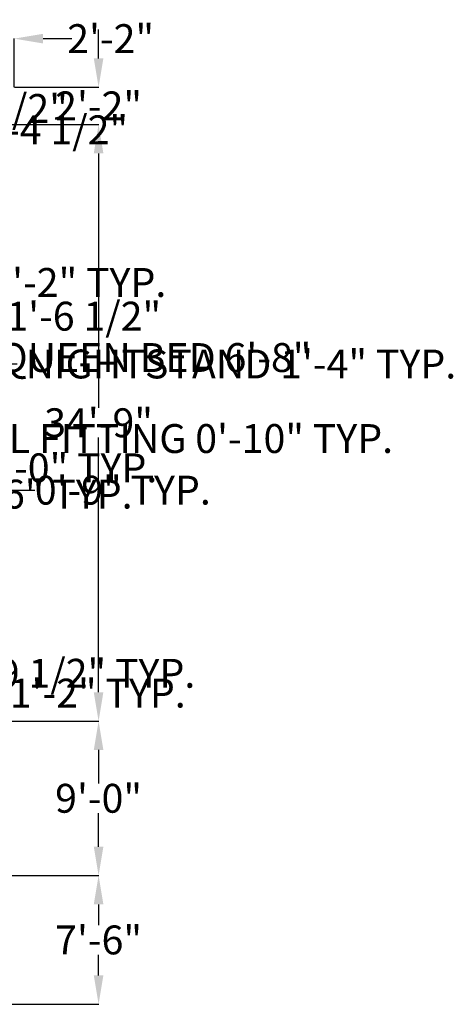
# Model space of a CAD drawing. Units: inches. Extents: x 1202 to 2101, y 998 to 1743.
# Tile 4 of 4: x 1798 to 2101, y 1054 to 1743. Entities that reach past the tile are written whole.
import ezdxf

# ---------------------------------------------------------------- set-up
doc = ezdxf.new("R2010")
doc.units = ezdxf.units.IN
doc.header["$MEASUREMENT"] = 0
doc.layers.add('A-ANNO-DIMS', color=2, linetype='Continuous', lineweight=18)
doc.styles.get("Standard").update_dxf_attribs({"font": 'arial.ttf'})
doc.dimstyles.get("Standard").update_dxf_attribs({"dimtxt": 20.18, "dimasz": 20.18, "dimexe": 0.18, "dimexo": 0.0625, "dimgap": 0.09, "dimtad": 0, "dimtih": 1, "dimtoh": 1, "dimdec": 0, "dimzin": 0, "dimdsep": 46, "dimlunit": 3, "dimtxsty": 'Standard', "dimcen": 0.09, "dimadec": 0, "dimazin": 0, "dimtfac": 1, "dimtdec": 0, "dimtofl": 0, "dimtmove": 0, "dimatfit": 3, "dimfxl": 1, "dimtolj": 1, "dimtzin": 0, "dimarcsym": 0})

# ---------------------------------------------------------------- blocks, each defined once
blk = doc.blocks.new('*D21')
at = {"layer": 'A-ANNO-DIMS', "color": 0, "lineweight": -2, "transparency": 16777216}
for p, q in [((1771.58, 1461.65), (1771.58, 1481.83)), ((1768.04, 1441.47), (1771.76, 1441.47)), ((1768.04, 1417.47), (1771.76, 1417.47)), ((1771.58, 1397.29), (1771.58, 1377.11))]:
    blk.add_line(p, q, dxfattribs=at)
at = {"layer": 'A-ANNO-DIMS', "color": 0, "transparency": 16777216}
for points in [[(1768.21, 1461.65), (1774.94, 1461.65), (1771.58, 1441.47)], [(1768.21, 1397.29), (1774.94, 1397.29), (1771.58, 1417.47)]]:
    blk.add_solid(points, dxfattribs=at)
at = {"layer": 'Defpoints', "color": 0, "transparency": 16777216}
for p in [(1767.98, 1441.47), (1771.58, 1441.47), (1767.98, 1417.47)]:
    blk.add_point(p, dxfattribs=at)
at = {"layer": 'A-ANNO-DIMS', "color": 0, "transparency": 16777216, "insert": (1771.58, 1429.47), "char_height": 20.18, "attachment_point": 5}
blk.add_mtext('\\A1;WINDOW 2\'-0" TYP.', dxfattribs=at)
blk = doc.blocks.new('*D22')
at = {"layer": 'A-ANNO-DIMS', "color": 0, "lineweight": -2, "transparency": 16777216}
for p, q in [((1738.8, 1413.87), (1718.62, 1413.87)), ((1758.98, 1417.4), (1758.98, 1413.69)), ((1767.98, 1417.4), (1767.98, 1413.69)), ((1788.16, 1413.87), (1808.34, 1413.87))]:
    blk.add_line(p, q, dxfattribs=at)
at = {"layer": 'A-ANNO-DIMS', "color": 0, "transparency": 16777216}
for points in [[(1738.8, 1417.23), (1738.8, 1410.5), (1758.98, 1413.87)], [(1788.16, 1417.23), (1788.16, 1410.5), (1767.98, 1413.87)]]:
    blk.add_solid(points, dxfattribs=at)
at = {"layer": 'Defpoints', "color": 0, "transparency": 16777216}
for p in [(1758.98, 1417.47), (1767.98, 1417.47), (1767.98, 1413.87)]:
    blk.add_point(p, dxfattribs=at)
at = {"layer": 'A-ANNO-DIMS', "color": 0, "transparency": 16777216, "insert": (1869.93, 1413.87), "char_height": 20.18, "attachment_point": 5}
blk.add_mtext('\\A1;0\'-9" TYP.', dxfattribs=at)
blk = doc.blocks.new('*D23')
at = {"layer": 'A-ANNO-DIMS', "color": 0, "lineweight": -2, "transparency": 16777216}
for p, q in [((1705.63, 1429.75), (1705.63, 1449.93)), ((1705.63, 1449.93), (1725.81, 1449.93)), ((1707.09, 1409.57), (1705.45, 1409.57)), ((1707.09, 1399.47), (1705.45, 1399.47)), ((1705.63, 1379.29), (1705.63, 1359.11))]:
    blk.add_line(p, q, dxfattribs=at)
at = {"layer": 'A-ANNO-DIMS', "color": 0, "transparency": 16777216}
for points in [[(1702.27, 1429.75), (1709, 1429.75), (1705.63, 1409.57)], [(1702.27, 1379.29), (1709, 1379.29), (1705.63, 1399.47)]]:
    blk.add_solid(points, dxfattribs=at)
at = {"layer": 'Defpoints', "color": 0, "transparency": 16777216}
for p in [(1705.63, 1409.57), (1707.15, 1409.57), (1707.15, 1399.47)]:
    blk.add_point(p, dxfattribs=at)
at = {"layer": 'A-ANNO-DIMS', "color": 0, "transparency": 16777216, "insert": (1896.68, 1449.93), "char_height": 20.18, "attachment_point": 5}
blk.add_mtext('\\A1;WALL FITTING 0\'-10" TYP.', dxfattribs=at)
blk = doc.blocks.new('*D24')
at = {"layer": 'A-ANNO-DIMS', "color": 0, "lineweight": -2, "transparency": 16777216}
for p, q in [((1686.97, 1411.09), (1666.79, 1411.09)), ((1707.15, 1409.64), (1707.15, 1411.27)), ((1713.22, 1409.64), (1713.22, 1411.27)), ((1733.4, 1411.09), (1753.58, 1411.09))]:
    blk.add_line(p, q, dxfattribs=at)
at = {"layer": 'A-ANNO-DIMS', "color": 0, "transparency": 16777216}
for points in [[(1686.97, 1414.45), (1686.97, 1407.73), (1707.15, 1411.09)], [(1733.4, 1414.45), (1733.4, 1407.73), (1713.22, 1411.09)]]:
    blk.add_solid(points, dxfattribs=at)
at = {"layer": 'Defpoints', "color": 0, "transparency": 16777216}
for p in [(1713.22, 1411.09), (1707.15, 1409.57), (1713.22, 1409.57)]:
    blk.add_point(p, dxfattribs=at)
at = {"layer": 'A-ANNO-DIMS', "color": 0, "transparency": 16777216, "insert": (1815.17, 1411.09), "char_height": 20.18, "attachment_point": 5}
blk.add_mtext('\\A1;0\'-6" TYP.', dxfattribs=at)
blk = doc.blocks.new('*D25')
at = {"layer": 'A-ANNO-DIMS', "color": 0, "lineweight": -2, "transparency": 16777216}
for p, q in [((1754.58, 1316.69), (1754.58, 1336.87)), ((1751.44, 1296.51), (1754.76, 1296.51)), ((1751.44, 1275.18), (1754.76, 1275.18)), ((1754.58, 1255), (1754.58, 1234.82))]:
    blk.add_line(p, q, dxfattribs=at)
at = {"layer": 'A-ANNO-DIMS', "color": 0, "transparency": 16777216}
for points in [[(1751.22, 1316.69), (1757.94, 1316.69), (1754.58, 1296.51)], [(1751.22, 1255), (1757.94, 1255), (1754.58, 1275.18)]]:
    blk.add_solid(points, dxfattribs=at)
at = {"layer": 'Defpoints', "color": 0, "transparency": 16777216}
for p in [(1751.38, 1296.51), (1754.58, 1296.51), (1751.38, 1275.18)]:
    blk.add_point(p, dxfattribs=at)
at = {"layer": 'A-ANNO-DIMS', "color": 0, "transparency": 16777216, "insert": (1754.58, 1285.85), "char_height": 20.18, "attachment_point": 5}
blk.add_mtext('\\A1;PILLOW SET 1\'-9 1/2" TYP.', dxfattribs=at)
blk = doc.blocks.new('*D26')
at = {"layer": 'A-ANNO-DIMS', "color": 0, "lineweight": -2, "transparency": 16777216}
for p, q in [((1737.22, 1275.12), (1737.22, 1271.8)), ((1751.38, 1275.12), (1751.38, 1271.8)), ((1717.04, 1271.98), (1696.86, 1271.98)), ((1771.56, 1271.98), (1791.74, 1271.98))]:
    blk.add_line(p, q, dxfattribs=at)
at = {"layer": 'A-ANNO-DIMS', "color": 0, "transparency": 16777216}
for points in [[(1717.04, 1275.35), (1717.04, 1268.62), (1737.22, 1271.98)], [(1771.56, 1275.35), (1771.56, 1268.62), (1751.38, 1271.98)]]:
    blk.add_solid(points, dxfattribs=at)
at = {"layer": 'Defpoints', "color": 0, "transparency": 16777216}
for p in [(1737.22, 1275.18), (1751.38, 1275.18), (1751.38, 1271.98)]:
    blk.add_point(p, dxfattribs=at)
at = {"layer": 'A-ANNO-DIMS', "color": 0, "transparency": 16777216, "insert": (1852.38, 1271.98), "char_height": 20.18, "attachment_point": 5}
blk.add_mtext('\\A1;1\'-2" TYP.', dxfattribs=at)
blk = doc.blocks.new('*D27')
at = {"layer": 'A-ANNO-DIMS', "color": 0, "lineweight": -2, "transparency": 16777216}
for p, q in [((1719.4, 1502.04), (1699.22, 1502.04)), ((1739.58, 1504.38), (1739.58, 1501.86)), ((1755.58, 1504.38), (1755.58, 1501.86)), ((1775.76, 1502.04), (1795.94, 1502.04))]:
    blk.add_line(p, q, dxfattribs=at)
at = {"layer": 'A-ANNO-DIMS', "color": 0, "transparency": 16777216}
for points in [[(1719.4, 1505.41), (1719.4, 1498.68), (1739.58, 1502.04)], [(1775.76, 1505.41), (1775.76, 1498.68), (1755.58, 1502.04)]]:
    blk.add_solid(points, dxfattribs=at)
at = {"layer": 'Defpoints', "color": 0, "transparency": 16777216}
for p in [(1739.58, 1504.44), (1755.58, 1504.44), (1755.58, 1502.04)]:
    blk.add_point(p, dxfattribs=at)
at = {"layer": 'A-ANNO-DIMS', "color": 0, "transparency": 16777216, "insert": (1952.58, 1502.04), "char_height": 20.18, "attachment_point": 5}
blk.add_mtext('\\A1;NIGHTSTAND 1\'-4" TYP.', dxfattribs=at)
blk = doc.blocks.new('*D28')
at = {"layer": 'A-ANNO-DIMS', "color": 0, "lineweight": -2, "transparency": 16777216}
for p, q in [((1757.98, 1538.86), (1757.98, 1559.04)), ((1757.98, 1559.04), (1778.16, 1559.04)), ((1755.64, 1518.68), (1758.16, 1518.68)), ((1755.64, 1504.44), (1758.16, 1504.44)), ((1757.98, 1484.26), (1757.98, 1464.08))]:
    blk.add_line(p, q, dxfattribs=at)
at = {"layer": 'A-ANNO-DIMS', "color": 0, "transparency": 16777216}
for points in [[(1754.62, 1538.86), (1761.34, 1538.86), (1757.98, 1518.68)], [(1754.62, 1484.26), (1761.34, 1484.26), (1757.98, 1504.44)]]:
    blk.add_solid(points, dxfattribs=at)
at = {"layer": 'Defpoints', "color": 0, "transparency": 16777216}
for p in [(1755.58, 1518.68), (1757.98, 1518.68), (1755.58, 1504.44)]:
    blk.add_point(p, dxfattribs=at)
at = {"layer": 'A-ANNO-DIMS', "color": 0, "transparency": 16777216, "insert": (1838.8, 1559.04), "char_height": 20.18, "attachment_point": 5}
blk.add_mtext('\\A1;1\'-2" TYP.', dxfattribs=at)
blk = doc.blocks.new('*D29')
at = {"layer": 'A-ANNO-DIMS', "color": 0, "lineweight": -2, "transparency": 16777216}
for p, q in [((1678.41, 1518.49), (1678.41, 1506.37)), ((1758.41, 1518.49), (1758.41, 1506.37)), ((1698.59, 1506.55), (1738.23, 1506.55)), ((1758.41, 1506.55), (1778.59, 1506.55))]:
    blk.add_line(p, q, dxfattribs=at)
at = {"layer": 'A-ANNO-DIMS', "color": 0, "transparency": 16777216}
for points in [[(1698.59, 1509.91), (1698.59, 1503.18), (1678.41, 1506.55)], [(1738.23, 1509.91), (1738.23, 1503.18), (1758.41, 1506.55)]]:
    blk.add_solid(points, dxfattribs=at)
at = {"layer": 'Defpoints', "color": 0, "transparency": 16777216}
for p in [(1678.41, 1518.55), (1758.41, 1518.55), (1758.41, 1506.55)]:
    blk.add_point(p, dxfattribs=at)
at = {"layer": 'A-ANNO-DIMS', "color": 0, "transparency": 16777216, "insert": (1892.42, 1506.55), "char_height": 20.18, "attachment_point": 5}
blk.add_mtext('\\A1;QUEEN BED 6\'-8"', dxfattribs=at)
blk = doc.blocks.new('*D37')
at = {"layer": 'A-ANNO-DIMS', "color": 0, "lineweight": -2, "transparency": 16777216}
for p, q in [((1628.63, 1659.71), (1628.63, 1665.93)), ((1648.81, 1665.75), (1649.15, 1665.75)), ((1669.33, 1659.71), (1669.33, 1665.93)), ((1669.33, 1665.75), (1689.51, 1665.75))]:
    blk.add_line(p, q, dxfattribs=at)
at = {"layer": 'A-ANNO-DIMS', "color": 0, "transparency": 16777216}
for points in [[(1648.81, 1669.11), (1648.81, 1662.39), (1628.63, 1665.75)], [(1649.15, 1669.11), (1649.15, 1662.39), (1669.33, 1665.75)]]:
    blk.add_solid(points, dxfattribs=at)
at = {"layer": 'Defpoints', "color": 0, "transparency": 16777216}
for p in [(1669.33, 1665.75), (1628.63, 1659.65), (1669.33, 1659.65)]:
    blk.add_point(p, dxfattribs=at)
at = {"layer": 'A-ANNO-DIMS', "color": 0, "transparency": 16777216, "insert": (1781.74, 1665.75), "char_height": 20.18, "attachment_point": 5}
blk.add_mtext('\\A1;DESK 3\'-4 1/2"', dxfattribs=at)
blk = doc.blocks.new('*D41')
at = {"layer": 'A-ANNO-DIMS', "color": 0, "lineweight": -2, "transparency": 16777216}
for p, q in [((1618.04, 1252.47), (1853.16, 1252.47)), ((1852.98, 1232.29), (1852.98, 1208.86)), ((1852.98, 1164.65), (1852.98, 1188.07)), ((1759.04, 1144.47), (1853.16, 1144.47))]:
    blk.add_line(p, q, dxfattribs=at)
at = {"layer": 'A-ANNO-DIMS', "color": 0, "transparency": 16777216}
for points in [[(1849.61, 1232.29), (1856.34, 1232.29), (1852.98, 1252.47)], [(1849.61, 1164.65), (1856.34, 1164.65), (1852.98, 1144.47)]]:
    blk.add_solid(points, dxfattribs=at)
at = {"layer": 'Defpoints', "color": 0, "transparency": 16777216}
for p in [(1617.98, 1252.47), (1852.98, 1252.47), (1758.98, 1144.47)]:
    blk.add_point(p, dxfattribs=at)
at = {"layer": 'A-ANNO-DIMS', "color": 0, "transparency": 16777216, "insert": (1852.98, 1198.47), "char_height": 20.18, "attachment_point": 5}
blk.add_mtext('\\A1;9\'-0"', dxfattribs=at)
blk = doc.blocks.new('*D42')
at = {"layer": 'A-ANNO-DIMS', "color": 0, "lineweight": -2, "transparency": 16777216}
for p, q in [((1768.04, 1669.47), (1853.16, 1669.47)), ((1852.98, 1649.29), (1852.98, 1471.37)), ((1852.98, 1272.65), (1852.98, 1450.57)), ((1618.04, 1252.47), (1853.16, 1252.47))]:
    blk.add_line(p, q, dxfattribs=at)
at = {"layer": 'A-ANNO-DIMS', "color": 0, "transparency": 16777216}
for points in [[(1849.61, 1649.29), (1856.34, 1649.29), (1852.98, 1669.47)], [(1849.61, 1272.65), (1856.34, 1272.65), (1852.98, 1252.47)]]:
    blk.add_solid(points, dxfattribs=at)
at = {"layer": 'Defpoints', "color": 0, "transparency": 16777216}
for p in [(1767.98, 1669.47), (1852.98, 1669.47), (1617.98, 1252.47)]:
    blk.add_point(p, dxfattribs=at)
at = {"layer": 'A-ANNO-DIMS', "color": 0, "transparency": 16777216, "insert": (1852.98, 1460.97), "char_height": 20.18, "attachment_point": 5}
blk.add_mtext('\\A1;34\'-9"', dxfattribs=at)
blk = doc.blocks.new('*D43')
at = {"layer": 'A-ANNO-DIMS', "color": 0, "lineweight": -2, "transparency": 16777216}
for p, q in [((1852.98, 1715.65), (1852.98, 1735.83)), ((1794.04, 1695.47), (1853.16, 1695.47)), ((1768.04, 1669.47), (1853.16, 1669.47)), ((1852.98, 1649.29), (1852.98, 1629.11))]:
    blk.add_line(p, q, dxfattribs=at)
at = {"layer": 'A-ANNO-DIMS', "color": 0, "transparency": 16777216}
for points in [[(1849.61, 1715.65), (1856.34, 1715.65), (1852.98, 1695.47)], [(1849.61, 1649.29), (1856.34, 1649.29), (1852.98, 1669.47)]]:
    blk.add_solid(points, dxfattribs=at)
at = {"layer": 'Defpoints', "color": 0, "transparency": 16777216}
for p in [(1793.98, 1695.47), (1852.98, 1695.47), (1767.98, 1669.47)]:
    blk.add_point(p, dxfattribs=at)
at = {"layer": 'A-ANNO-DIMS', "color": 0, "transparency": 16777216, "insert": (1852.98, 1682.47), "char_height": 20.18, "attachment_point": 5}
blk.add_mtext('\\A1;2\'-2"', dxfattribs=at)
blk = doc.blocks.new('*D45')
at = {"layer": 'A-ANNO-DIMS', "color": 0, "lineweight": -2, "transparency": 16777216}
for p, q in [((1747.8, 1729.47), (1727.62, 1729.47)), ((1767.98, 1669.53), (1767.98, 1729.65)), ((1793.98, 1695.53), (1793.98, 1729.65)), ((1814.16, 1729.47), (1834.34, 1729.47))]:
    blk.add_line(p, q, dxfattribs=at)
at = {"layer": 'A-ANNO-DIMS', "color": 0, "transparency": 16777216}
for points in [[(1747.8, 1732.83), (1747.8, 1726.1), (1767.98, 1729.47)], [(1814.16, 1732.83), (1814.16, 1726.1), (1793.98, 1729.47)]]:
    blk.add_solid(points, dxfattribs=at)
at = {"layer": 'Defpoints', "color": 0, "transparency": 16777216}
for p in [(1793.98, 1729.47), (1793.98, 1695.47), (1767.98, 1669.47)]:
    blk.add_point(p, dxfattribs=at)
at = {"layer": 'A-ANNO-DIMS', "color": 0, "transparency": 16777216, "insert": (1861.42, 1729.47), "char_height": 20.18, "attachment_point": 5}
blk.add_mtext('\\A1;2\'-2"', dxfattribs=at)
blk = doc.blocks.new('*D46')
at = {"layer": 'A-ANNO-DIMS', "color": 0, "lineweight": -2, "transparency": 16777216}
for p, q in [((1759.04, 1144.47), (1853.16, 1144.47)), ((1852.98, 1124.29), (1852.98, 1109.86)), ((1852.98, 1074.65), (1852.98, 1089.07)), ((1759.04, 1054.47), (1853.16, 1054.47))]:
    blk.add_line(p, q, dxfattribs=at)
at = {"layer": 'A-ANNO-DIMS', "color": 0, "transparency": 16777216}
for points in [[(1849.61, 1124.29), (1856.34, 1124.29), (1852.98, 1144.47)], [(1849.61, 1074.65), (1856.34, 1074.65), (1852.98, 1054.47)]]:
    blk.add_solid(points, dxfattribs=at)
at = {"layer": 'Defpoints', "color": 0, "transparency": 16777216}
for p in [(1758.98, 1144.47), (1852.98, 1144.47), (1758.98, 1054.47)]:
    blk.add_point(p, dxfattribs=at)
at = {"layer": 'A-ANNO-DIMS', "color": 0, "transparency": 16777216, "insert": (1852.98, 1099.47), "char_height": 20.18, "attachment_point": 5}
blk.add_mtext('\\A1;7\'-6"', dxfattribs=at)
blk = doc.blocks.new('*D48')
at = {"layer": 'A-ANNO-DIMS', "color": 0, "lineweight": -2, "transparency": 16777216}
for p, q in [((1668.02, 1680.65), (1647.84, 1680.65)), ((1647.84, 1680.65), (1647.84, 1660.47)), ((1647.74, 1603.67), (1647.92, 1603.67)), ((1647.83, 1603.58), (1647.83, 1603.76))]:
    blk.add_line(p, q, dxfattribs=at)
at = {"layer": 'A-ANNO-DIMS', "color": 0, "transparency": 16777216}
blk.add_solid([(1644.47, 1660.47), (1651.2, 1660.47), (1647.84, 1640.29)], dxfattribs=at)
at = {"layer": 'Defpoints', "color": 0, "transparency": 16777216}
for p in [(1647.84, 1640.29), (1647.83, 1603.67)]:
    blk.add_point(p, dxfattribs=at)
at = {"layer": 'A-ANNO-DIMS', "color": 0, "transparency": 16777216, "insert": (1749.95, 1680.65), "char_height": 20.18, "attachment_point": 5}
blk.add_mtext('\\A1;2X R3\'-0 1/2"', dxfattribs=at)
blk = doc.blocks.new('*D50')
at = {"layer": 'A-ANNO-DIMS', "color": 0, "lineweight": -2, "transparency": 16777216}
for p, q in [((1712.91, 1535.47), (1705.73, 1516.61)), ((1733.09, 1535.47), (1712.91, 1535.47)), ((1691.93, 1480.57), (1692.11, 1480.57)), ((1692.02, 1480.48), (1692.02, 1480.66))]:
    blk.add_line(p, q, dxfattribs=at)
at = {"layer": 'A-ANNO-DIMS', "color": 0, "transparency": 16777216}
blk.add_solid([(1702.59, 1517.81), (1708.88, 1515.41), (1698.56, 1497.75)], dxfattribs=at)
at = {"layer": 'Defpoints', "color": 0, "transparency": 16777216}
for p in [(1698.56, 1497.75), (1692.02, 1480.57)]:
    blk.add_point(p, dxfattribs=at)
at = {"layer": 'A-ANNO-DIMS', "color": 0, "transparency": 16777216, "insert": (1815.26, 1535.47), "char_height": 20.18, "attachment_point": 5}
blk.add_mtext('\\A1;4X R1\'-6 1/2"', dxfattribs=at)

msp = doc.modelspace()

# ---------------------------------------------------------------- dimensions: what is measured, and where the dimension line sits
at = {"layer": 'A-ANNO-DIMS'}
dim = msp.add_linear_dim(base=(1793.98, 1729.47), p1=(1767.98, 1669.47), p2=(1793.98, 1695.47), dimstyle='Standard', override={"dimdec": 1, "dimlfac": 1, "dimrnd": 0, "dimzin": 1, "dimdsep": 46, "dimlunit": 4, "dimfrac": 2}, dxfattribs=at)
dim.commit()
dim.dimension.update_dxf_attribs({"geometry": '*D45', "text_midpoint": (1861.42, 1729.47)})
for base, p1, p2, picture, middle in [((1852.98, 1695.47), (1767.98, 1669.47), (1793.98, 1695.47), '*D43', (1852.98, 1682.47)), ((1852.98, 1669.47), (1617.98, 1252.47), (1767.98, 1669.47), '*D42', (1852.98, 1460.97)), ((1852.98, 1252.47), (1758.98, 1144.47), (1617.98, 1252.47), '*D41', (1852.98, 1198.47)), ((1852.98, 1144.47), (1758.98, 1054.47), (1758.98, 1144.47), '*D46', (1852.98, 1099.47))]:
    dim = msp.add_linear_dim(base=base, p1=p1, p2=p2, angle=90, dimstyle='Standard', override={"dimdec": 1, "dimlfac": 1, "dimrnd": 0, "dimzin": 1, "dimdsep": 46, "dimlunit": 4, "dimfrac": 2}, dxfattribs=at)
    dim.commit()
    dim.dimension.update_dxf_attribs({"geometry": picture, "text_midpoint": middle})
for center, mpoint, text, picture, middle in [((1647.83, 1603.67), (1647.84, 1640.29), '2X <>', '*D48', (1749.95, 1680.65)), ((1692.02, 1480.57), (1698.56, 1497.75), '4X <>', '*D50', (1815.26, 1535.47))]:
    dim = msp.add_radius_dim(center=center, mpoint=mpoint, text=text, dimstyle='Standard', override={"dimdec": 1, "dimlfac": 1, "dimrnd": 0, "dimzin": 1, "dimdsep": 46, "dimlunit": 4, "dimfrac": 2}, dxfattribs=at)
    dim.commit()
    dim.dimension.update_dxf_attribs({"geometry": picture, "text_midpoint": middle})
for base, p1, p2, text, picture, middle in [((1669.33, 1665.75), (1628.63, 1659.65), (1669.33, 1659.65), 'DESK <>', '*D37', (1781.74, 1665.75)), ((1758.41, 1506.55), (1678.41, 1518.55), (1758.41, 1518.55), 'QUEEN BED <>', '*D29', (1892.42, 1506.55)), ((1755.58, 1502.04), (1739.58, 1504.44), (1755.58, 1504.44), 'NIGHTSTAND <> TYP.', '*D27', (1952.58, 1502.04)), ((1713.22, 1411.09), (1707.15, 1409.57), (1713.22, 1409.57), '<> TYP.', '*D24', (1815.17, 1411.09)), ((1767.98, 1413.87), (1758.98, 1417.47), (1767.98, 1417.47), '<> TYP.', '*D22', (1869.93, 1413.87)), ((1751.38, 1271.98), (1737.22, 1275.18), (1751.38, 1275.18), '<> TYP.', '*D26', (1852.38, 1271.98))]:
    dim = msp.add_linear_dim(base=base, p1=p1, p2=p2, text=text, dimstyle='Standard', override={"dimdec": 1, "dimlfac": 1, "dimrnd": 0, "dimzin": 1, "dimdsep": 46, "dimlunit": 4, "dimfrac": 2}, dxfattribs=at)
    dim.commit()
    dim.dimension.update_dxf_attribs({"geometry": picture, "text_midpoint": middle})
for base, p1, p2, text, picture, middle in [((1757.98, 1518.68), (1755.58, 1504.44), (1755.58, 1518.68), '<> TYP.', '*D28', (1838.8, 1559.04)), ((1705.63, 1409.57), (1707.15, 1399.47), (1707.15, 1409.57), 'WALL FITTING <> TYP.', '*D23', (1896.68, 1449.93)), ((1771.58, 1441.47), (1767.98, 1417.47), (1767.98, 1441.47), 'WINDOW <> TYP.', '*D21', (1771.58, 1429.47)), ((1754.58, 1296.51), (1751.38, 1275.18), (1751.38, 1296.51), 'PILLOW SET <> TYP.', '*D25', (1754.58, 1285.85))]:
    dim = msp.add_linear_dim(base=base, p1=p1, p2=p2, angle=90, text=text, dimstyle='Standard', override={"dimdec": 1, "dimlfac": 1, "dimrnd": 0, "dimzin": 1, "dimdsep": 46, "dimlunit": 4, "dimfrac": 2}, dxfattribs=at)
    dim.commit()
    dim.dimension.update_dxf_attribs({"geometry": picture, "text_midpoint": middle})

doc.saveas('drawing.dxf')
